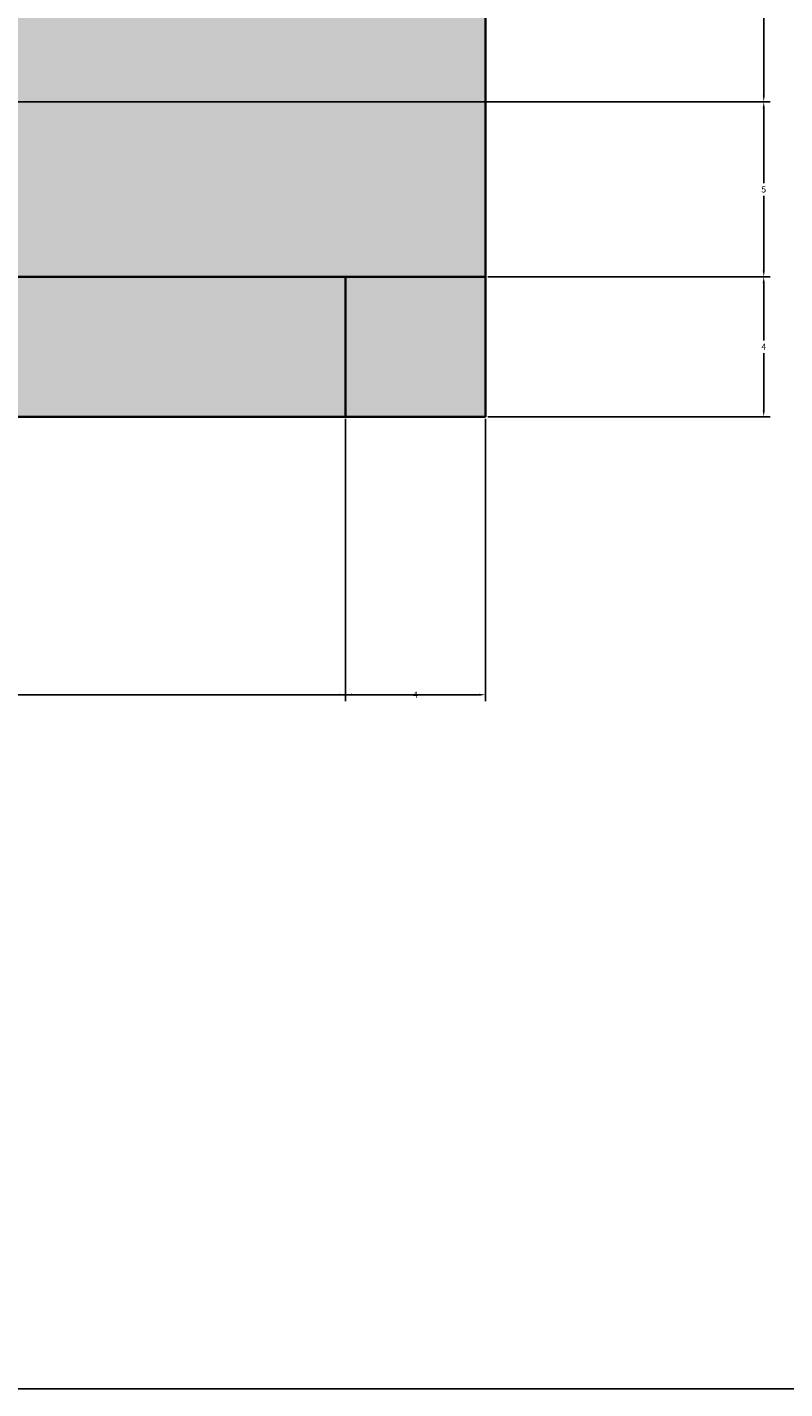
# Model space of a CAD drawing. Units: inches. Extents: x 4508 to 4723, y 847 to 1020.
# Tile 23 of 32: x 4681 to 4703, y 847 to 886. Entities that reach past the tile are written whole.
import ezdxf

# ---------------------------------------------------------------- set-up
doc = ezdxf.new("R2010")
doc.units = ezdxf.units.IN
for name, color, linetype, lineweight in [('A-ANNO-DIMS', 2, 'Continuous', 18), ('A-ANNO-TTLB', 7, 'Continuous', 25), ('A-WALL', 7, 'Continuous', 35), ('A-WALL-PATT', 254, 'Continuous', 13)]:
    doc.layers.add(name, color=color, linetype=linetype, lineweight=lineweight)
doc.styles.get("Standard").update_dxf_attribs({"font": 'arial.ttf'})
doc.dimstyles.get("Standard").update_dxf_attribs({"dimtxt": 0.18, "dimasz": 0.18, "dimexe": 0.18, "dimexo": 0.0625, "dimgap": 0.09, "dimtad": 0, "dimtih": 1, "dimtoh": 1, "dimdec": 4, "dimzin": 0, "dimdsep": 46, "dimtxsty": 'Standard', "dimcen": 0.09, "dimadec": 0, "dimazin": 0, "dimtfac": 1, "dimtdec": 4, "dimtofl": 0, "dimtmove": 0, "dimatfit": 3, "dimfxl": 1, "dimtolj": 1, "dimtzin": 0, "dimarcsym": 0})

# ---------------------------------------------------------------- blocks, each defined once
blk = doc.blocks.new('*D2')
at = {"layer": 'A-ANNO-DIMS', "color": 0, "lineweight": -2, "transparency": 16777216}
for p, q in [((4540.994, 874.684), (4540.994, 866.617)), ((4693.994, 874.684), (4693.994, 866.617)), ((4541.174, 866.797), (4617.213, 866.797)), ((4693.814, 866.797), (4617.774, 866.797))]:
    blk.add_line(p, q, dxfattribs=at)
at = {"layer": 'A-ANNO-DIMS', "color": 0, "lineweight": 9, "transparency": 16777216}
for points in [[(4541.174, 866.827), (4541.174, 866.767), (4540.994, 866.797)], [(4693.814, 866.827), (4693.814, 866.767), (4693.994, 866.797)]]:
    blk.add_solid(points, dxfattribs=at)
at = {"layer": 'Defpoints', "color": 0, "lineweight": 9, "transparency": 16777216}
for p in [(4540.994, 874.747), (4693.994, 874.747), (4693.994, 866.797)]:
    blk.add_point(p, dxfattribs=at)
at = {"layer": 'A-ANNO-DIMS', "color": 0, "transparency": 16777216, "insert": (4617.494, 866.797), "char_height": 0.18, "attachment_point": 5}
blk.add_mtext('\\A1;153', dxfattribs=at)
blk = doc.blocks.new('*D12')
at = {"layer": 'A-ANNO-DIMS', "color": 0, "lineweight": -2, "transparency": 16777216}
for p, q in [((4689.994, 874.684), (4689.994, 866.617)), ((4693.994, 874.684), (4693.994, 866.617)), ((4690.174, 866.797), (4691.842, 866.797)), ((4693.814, 866.797), (4692.146, 866.797))]:
    blk.add_line(p, q, dxfattribs=at)
at = {"layer": 'A-ANNO-DIMS', "color": 0, "lineweight": 9, "transparency": 16777216}
for points in [[(4690.174, 866.827), (4690.174, 866.767), (4689.994, 866.797)], [(4693.814, 866.827), (4693.814, 866.767), (4693.994, 866.797)]]:
    blk.add_solid(points, dxfattribs=at)
at = {"layer": 'Defpoints', "color": 0, "lineweight": 9, "transparency": 16777216}
for p in [(4689.994, 874.747), (4693.994, 874.747), (4693.994, 866.797)]:
    blk.add_point(p, dxfattribs=at)
at = {"layer": 'A-ANNO-DIMS', "color": 0, "transparency": 16777216, "insert": (4691.994, 866.797), "char_height": 0.18, "attachment_point": 5}
blk.add_mtext('\\A1;4', dxfattribs=at)
blk = doc.blocks.new('*D13')
at = {"layer": 'A-ANNO-DIMS', "color": 0, "lineweight": -2, "transparency": 16777216}
for p, q in [((4669.325, 973.916), (4669.325, 866.617)), ((4689.994, 874.684), (4689.994, 866.617)), ((4669.505, 866.797), (4679.264, 866.797)), ((4689.814, 866.797), (4680.054, 866.797))]:
    blk.add_line(p, q, dxfattribs=at)
at = {"layer": 'A-ANNO-DIMS', "color": 0, "lineweight": 9, "transparency": 16777216}
for points in [[(4669.505, 866.827), (4669.505, 866.767), (4669.325, 866.797)], [(4689.814, 866.827), (4689.814, 866.767), (4689.994, 866.797)]]:
    blk.add_solid(points, dxfattribs=at)
at = {"layer": 'Defpoints', "color": 0, "lineweight": 9, "transparency": 16777216}
for p in [(4669.325, 973.978), (4689.994, 874.747), (4689.994, 866.797)]:
    blk.add_point(p, dxfattribs=at)
at = {"layer": 'A-ANNO-DIMS', "color": 0, "transparency": 16777216, "insert": (4679.659, 866.797), "char_height": 0.18, "attachment_point": 5}
blk.add_mtext('\\A1;20.67', dxfattribs=at)
blk = doc.blocks.new('*D16')
at = {"layer": 'A-ANNO-DIMS', "color": 0, "lineweight": -2, "transparency": 16777216}
for p, q in [((4694.056279, 878.746874), (4702.123779, 878.746874)), ((4701.943779, 878.566874), (4701.943779, 876.926874)), ((4701.943779, 874.926874), (4701.943779, 876.566874)), ((4694.056279, 874.746874), (4702.123779, 874.746874))]:
    blk.add_line(p, q, dxfattribs=at)
at = {"layer": 'A-ANNO-DIMS', "color": 0, "lineweight": 9, "transparency": 16777216}
for points in [[(4701.913779, 878.566874), (4701.973779, 878.566874), (4701.943779, 878.746874)], [(4701.913779, 874.926874), (4701.973779, 874.926874), (4701.943779, 874.746874)]]:
    blk.add_solid(points, dxfattribs=at)
at = {"layer": 'Defpoints', "color": 0, "lineweight": 9, "transparency": 16777216}
for p in [(4693.993779, 878.746874), (4701.943779, 878.746874), (4693.993779, 874.746874)]:
    blk.add_point(p, dxfattribs=at)
at = {"layer": 'A-ANNO-DIMS', "color": 0, "transparency": 16777216, "insert": (4701.943779, 876.746874), "char_height": 0.18, "attachment_point": 5}
blk.add_mtext('\\A1;4', dxfattribs=at)
blk = doc.blocks.new('*D17')
at = {"layer": 'A-ANNO-DIMS', "color": 0, "lineweight": -2, "transparency": 16777216}
for p, q in [((4671.869, 883.747), (4702.124, 883.747)), ((4701.944, 883.567), (4701.944, 881.428)), ((4701.944, 878.927), (4701.944, 881.065)), ((4694.056, 878.747), (4702.124, 878.747))]:
    blk.add_line(p, q, dxfattribs=at)
at = {"layer": 'A-ANNO-DIMS', "color": 0, "lineweight": 9, "transparency": 16777216}
for points in [[(4701.914, 883.567), (4701.974, 883.567), (4701.944, 883.747)], [(4701.914, 878.927), (4701.974, 878.927), (4701.944, 878.747)]]:
    blk.add_solid(points, dxfattribs=at)
at = {"layer": 'Defpoints', "color": 0, "lineweight": 9, "transparency": 16777216}
for p in [(4671.806, 883.747), (4701.944, 883.747), (4693.994, 878.747)]:
    blk.add_point(p, dxfattribs=at)
at = {"layer": 'A-ANNO-DIMS', "color": 0, "transparency": 16777216, "insert": (4701.944, 881.247), "char_height": 0.18, "attachment_point": 5}
blk.add_mtext('\\A1;5', dxfattribs=at)
blk = doc.blocks.new('*D18')
at = {"layer": 'A-ANNO-DIMS', "color": 0, "lineweight": -2, "transparency": 16777216}
for p, q in [((4671.119, 901.747), (4702.124, 901.747)), ((4701.944, 901.567), (4701.944, 892.929)), ((4701.944, 883.927), (4701.944, 892.565)), ((4671.869, 883.747), (4702.124, 883.747))]:
    blk.add_line(p, q, dxfattribs=at)
at = {"layer": 'A-ANNO-DIMS', "color": 0, "lineweight": 9, "transparency": 16777216}
for points in [[(4701.914, 901.567), (4701.974, 901.567), (4701.944, 901.747)], [(4701.914, 883.927), (4701.974, 883.927), (4701.944, 883.747)]]:
    blk.add_solid(points, dxfattribs=at)
at = {"layer": 'Defpoints', "color": 0, "lineweight": 9, "transparency": 16777216}
for p in [(4671.056, 901.747), (4701.944, 901.747), (4671.806, 883.747)]:
    blk.add_point(p, dxfattribs=at)
at = {"layer": 'A-ANNO-DIMS', "color": 0, "transparency": 16777216, "insert": (4701.944, 892.747), "char_height": 0.18, "attachment_point": 5}
blk.add_mtext('\\A1;18', dxfattribs=at)

msp = doc.modelspace()

# ---------------------------------------------------------------- hatches: boundary and pattern name
at = {"layer": 'A-WALL-PATT', "transparency": 33554508}
h = msp.add_hatch(color=256, dxfattribs=at)
h.dxf.hatch_style = 1
h.paths.add_polyline_path([(4661.6706, 954.043, -0.3739004), (4658.5765, 957.6021, -1), (4665.7646, 957.6021, -0.3739004), (4662.6706, 954.043), (4662.6706, 944.4021, -0.2114781), (4670.3062, 945.0869), (4670.3062, 968.0592, -0.4632086), (4663.3246, 973.9783, -0.4632086), (4670.3062, 979.8975), (4670.3062, 994.7469), (4588.9938, 994.7469), (4588.9938, 904.7469), (4657.9938, 904.7469), (4657.9938, 886.7469), (4549.9938, 886.7469), (4549.9938, 878.7469), (4693.9938, 878.7469), (4693.9938, 994.7469), (4671.8062, 994.7469), (4671.8062, 979.4411, -0.2941682), (4675.3246, 973.9783, -0.2941682), (4671.8062, 968.5156), (4671.8062, 944.4278, -0.2741114), (4676.7298, 936.1217, -0.2741114), (4671.8062, 927.8155), (4671.8062, 907.6998, -0.3779645), (4677.0562, 901.7469, -0.3779645), (4671.8062, 895.7939), (4671.8062, 883.7469), (4670.3062, 883.7469), (4670.3062, 895.7939, -0.3779645), (4665.0562, 901.7469, -0.3779645), (4670.3062, 907.6998), (4670.3062, 927.1564, -0.2114781), (4662.6706, 927.8412), (4662.6706, 918.2003, -0.3739004), (4665.7646, 914.6412, -1), (4658.5765, 914.6412, -0.3739004), (4661.6706, 918.2003), (4661.6706, 928.4807, -0.2391825), (4657.7936, 936.1217, -0.2391825), (4661.6706, 943.7626)])
at = {"layer": 'A-WALL-PATT', "transparency": 33554556}
h = msp.add_hatch(color=256, dxfattribs=at)
h.dxf.hatch_style = 1
h.paths.add_polyline_path([(4689.9938, 878.7469), (4549.9938, 878.7469), (4549.9938, 874.7469), (4689.9938, 874.7469)])
h = msp.add_hatch(color=256, dxfattribs=at)
h.dxf.hatch_style = 1
h.paths.add_polyline_path([(4693.9938, 878.7469), (4689.9938, 878.7469), (4689.9938, 874.7469), (4693.9938, 874.7469)])

# ---------------------------------------------------------------- linework, layer by layer
at = {"layer": 'A-ANNO-TTLB'}
msp.add_lwpolyline([(4508.3867, 1019.9118), (4722.9774, 1019.9118), (4722.9774, 846.9535), (4508.3867, 846.9535)], close=True, dxfattribs=at)
at = {"layer": 'A-WALL'}
for p, q in [((4693.9938, 994.7469), (4693.9938, 874.7469)), ((4693.9938, 878.7469), (4549.9938, 878.7469)), ((4689.9938, 878.7469), (4689.9938, 874.7469)), ((4693.9938, 874.7469), (4549.9938, 874.7469))]:
    msp.add_line(p, q, dxfattribs=at)

# ---------------------------------------------------------------- dimensions: what is measured, and where the dimension line sits
at = {"layer": 'A-ANNO-DIMS'}
for base, p1, p2, override, picture, middle in [((4689.9938, 866.7969), (4669.3246, 973.9783), (4689.9938, 874.7469), {"dimdec": 2, "dimlfac": 1, "dimrnd": 0, "dimzin": 0, "dimdsep": 46, "dimlunit": 2}, '*D13', (4679.6592, 866.7969)), ((4693.9938, 866.7969), (4540.9938, 874.7469), (4693.9938, 874.7469), {"dimdec": 0, "dimlfac": 1, "dimrnd": 0, "dimzin": 0, "dimdsep": 46, "dimlunit": 2}, '*D2', (4617.4938, 866.7969)), ((4693.9938, 866.7969), (4689.9938, 874.7469), (4693.9938, 874.7469), {"dimdec": 0, "dimlfac": 1, "dimrnd": 0, "dimzin": 0, "dimdsep": 46, "dimlunit": 2}, '*D12', (4691.9938, 866.7969))]:
    dim = msp.add_linear_dim(base=base, p1=p1, p2=p2, dimstyle='Standard', override=override, dxfattribs=at)
    dim.commit()
    dim.dimension.update_dxf_attribs({"geometry": picture, "text_midpoint": middle})
for base, p1, p2, picture, middle in [((4701.9438, 901.7469), (4671.8062, 883.7469), (4671.0562, 901.7469), '*D18', (4701.9438, 892.7469)), ((4701.9438, 883.7469), (4693.9938, 878.7469), (4671.8062, 883.7469), '*D17', (4701.9438, 881.2469)), ((4701.9438, 878.7469), (4693.9938, 874.7469), (4693.9938, 878.7469), '*D16', (4701.9438, 876.7469))]:
    dim = msp.add_linear_dim(base=base, p1=p1, p2=p2, angle=90, dimstyle='Standard', override={"dimdec": 0, "dimlfac": 1, "dimrnd": 0, "dimzin": 0, "dimdsep": 46, "dimlunit": 2}, dxfattribs=at)
    dim.commit()
    dim.dimension.update_dxf_attribs({"geometry": picture, "text_midpoint": middle})

doc.saveas('drawing.dxf')
